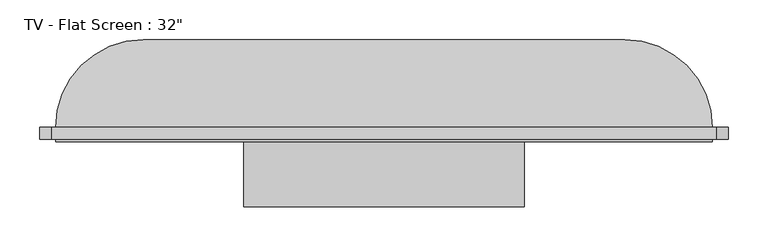
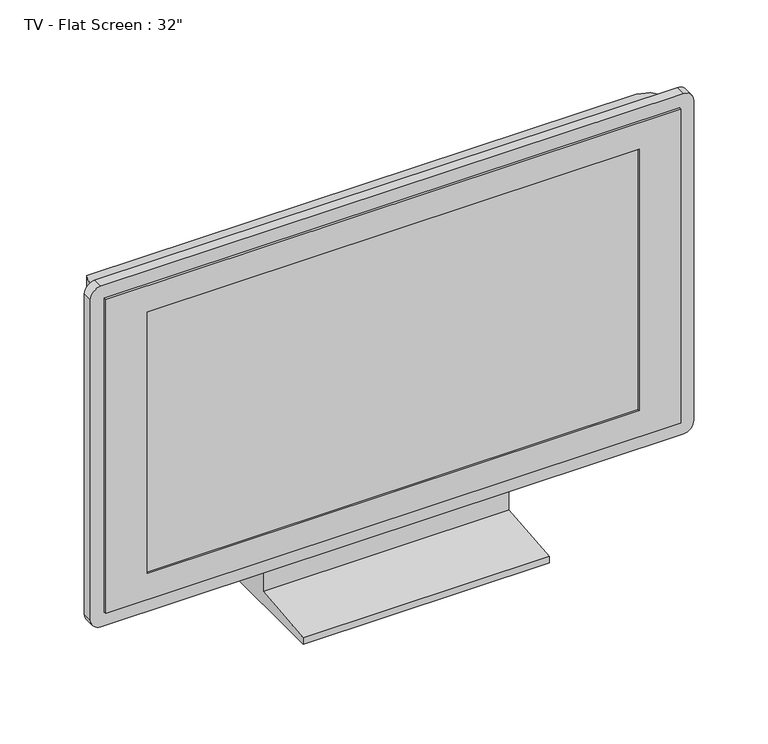
"""IFC4 building model written with IfcOpenShell, lengths in millimetres: furniture geometry."""

from ifc_helpers import new_model, si_unit, point, frame, frame_2d, origin, place, context, project, spatial, polyline, circle_curve, ellipse_curve, trimmed, segment, composite_curve, outline, extrude, faceted_brep, source, transform, mapped, element, save
from ifc_brep_helpers import plane_surface, cylinder_surface, advanced_brep


def furniture_56245f3a(model_context):
    return source(origin(), model_context, "Body", "SolidModel", [
        extrude(outline(polyline([(-51.4613764, 80.0), (-1.4613764, 80.0), (48.5386236, 0.0), (-151.4613764, 0.0), (-151.4613764, 10.0), (-51.4613764, 20.0), (-51.4613764, 80.0)])), frame((-180.4346678, 0.0, 0.0), z_axis=(1.0, 0.0, 0.0), x_axis=(0.0, 1.0, 0.0)), (0.0, 0.0, 1.0), 352.9803073),
        faceted_brep([(409.0357931, -69.4613764, 557.1392838), (-416.9248214, -69.4613764, 557.1392838), (-416.9248214, -69.4613764, 80.0), (409.0357931, -69.4613764, 80.0), (-356.9248214, -69.4613764, 517.1392838), (349.0357931, -69.4613764, 517.1392838), (349.0357931, -69.4613764, 120.0), (-356.9248214, -69.4613764, 120.0), (409.0357931, -51.4613764, 557.1392838), (409.0357931, -51.4613764, 80.0), (-416.9248214, -51.4613764, 80.0), (-416.9248214, -51.4613764, 557.1392838), (-356.9248214, -66.4613764, 517.1392838), (-356.9248214, -66.4613764, 120.0), (349.0357931, -66.4613764, 120.0), (349.0357931, -66.4613764, 517.1392838)], [[[0, 1, 2, 3], [4, 5, 6, 7]], [[8, 9, 10, 11]], [[1, 0, 8, 11]], [[2, 1, 11, 10]], [[3, 2, 10, 9]], [[0, 3, 9, 8]], [[12, 13, 14, 15]], [[12, 15, 5, 4]], [[15, 14, 6, 5]], [[14, 13, 7, 6]], [[13, 12, 4, 7]]]),
        extrude(outline(composite_curve([segment(polyline([(577.1392838, 414.0357931), (577.1392838, -421.9248214)]), True, "CONTINUOUS"), segment(trimmed(circle_curve(frame_2d((562.1392838, -421.9248214)), 15.0), [point((577.1392838, -421.9248214))], [point((562.1392838, -436.9248214))], False, "CARTESIAN"), True, "CONTINUOUS"), segment(polyline([(562.1392838, -436.9248214), (75.0, -436.9248214)]), True, "CONTINUOUS"), segment(trimmed(circle_curve(frame_2d((75.0, -421.9248214)), 15.0), [point((75.0, -436.9248214))], [point((60.0, -421.9248214))], False, "CARTESIAN"), True, "CONTINUOUS"), segment(polyline([(60.0, -421.9248214), (60.0, 414.0357931)]), True, "CONTINUOUS"), segment(trimmed(circle_curve(frame_2d((75.0, 414.0357931)), 15.0), [point((60.0, 414.0357931))], [point((75.0, 429.0357931))], False, "CARTESIAN"), True, "CONTINUOUS"), segment(polyline([(75.0, 429.0357931), (562.1392838, 429.0357931)]), True, "CONTINUOUS"), segment(trimmed(circle_curve(frame_2d((562.1392838, 414.0357931)), 15.0), [point((562.1392838, 429.0357931))], [point((577.1392838, 414.0357931))], False, "CARTESIAN"), True, "CONTINUOUS")], self_intersect=False), holes=[polyline([(557.1392838, 409.0357931), (80.0, 409.0357931), (80.0, -416.9248214), (557.1392838, -416.9248214), (557.1392838, 409.0357931)])]), frame((0.0, -66.4613764, 0.0), z_axis=(0.0, 1.0, 0.0), x_axis=(0.0, 0.0, 1.0)), (0.0, 0.0, 1.0), 15.0),
        advanced_brep(
        [(-416.9248214, -51.4613764, 80.0), (409.0357931, -51.4613764, 80.0), (409.0357931, -51.4613764, 557.1392838), (-416.9248214, -51.4613764, 557.1392838), (299.0357931, 58.5386236, 80.0), (-306.9248214, 58.5386236, 80.0), (-306.9248214, 58.5386236, 447.1392838), (299.0357931, 58.5386236, 447.1392838)],
        [
            (0, 1),
            (1, 2),
            (2, 3),
            (3, 0),
            (4, 5),
            (5, 6),
            (6, 7),
            (7, 4),
            (0, 5, circle_curve(frame((-306.9248214, -51.4613764, 80.0), z_axis=(0.0, 0.0, -1.0), x_axis=(-1.0, 0.0, 0.0)), 110.0)),
            (4, 1, circle_curve(frame((299.0357931, -51.4613764, 80.0), z_axis=(0.0, 0.0, -1.0), x_axis=(1.0, 0.0, 0.0)), 110.0)),
            (7, 2, ellipse_curve(frame((299.0357931, -51.4613764, 447.1392838), z_axis=(0.7071067811865475, 0.0, -0.7071067811865475), x_axis=(0.7071067811865474, 0.0, 0.7071067811865476)), 155.5634919, 110.0)),
            (6, 3, ellipse_curve(frame((-306.9248214, -51.4613764, 447.1392838), z_axis=(0.7071067811865475, 0.0, 0.7071067811865475), x_axis=(-0.7071067811865476, 0.0, 0.7071067811865474)), 155.5634919, 110.0)),
        ],
        [
            plane_surface(frame((-416.9248214, -51.4613764, 557.1392838), z_axis=(0.0, -1.0, 0.0), x_axis=(-1.0, 0.0, 0.0))),
            plane_surface(frame((-416.9248214, 58.5386236, 557.1392838), z_axis=(0.0, 1.0, 0.0), x_axis=(1.0, 0.0, 0.0))),
            plane_surface(frame((-416.9248214, -51.4613764, 80.0), z_axis=(0.0, 0.0, -1.0), x_axis=(0.0, 1.0, 0.0))),
            cylinder_surface(frame((299.0357931, -51.4613764, 80.0), z_axis=(0.0, 0.0, 1.0), x_axis=(1.0, 0.0, 0.0)), 110.0),
            cylinder_surface(frame((409.0357931, -51.4613764, 447.1392838), z_axis=(-1.0, 0.0, 0.0), x_axis=(0.0, 0.0, 1.0)), 110.0),
            cylinder_surface(frame((-306.9248214, -51.4613764, 557.1392838), z_axis=(0.0, 0.0, -1.0), x_axis=(-1.0, 0.0, 0.0)), 110.0),
        ],
        [
            (0, [[1, 2, 3, 4]]),
            (1, [[5, 6, 7, 8]]),
            (2, [[-1, 9, -5, 10]]),
            (3, [[11, -2, -10, -8]]),
            (4, [[-11, -7, 12, -3]]),
            (5, [[-12, -6, -9, -4]]),
        ],
    ),
    ])


if __name__ == "__main__":
    model = new_model("IFC4")
    model_context = context("Model", 3, world=origin())
    ifc_project = project(units=[si_unit("LENGTHUNIT", "METRE", prefix="MILLI")], contexts=[model_context])
    site = spatial("IfcSite", under=ifc_project)
    building = spatial("IfcBuilding", under=site)
    placement = place(None, origin())
    furniture_shape = furniture_56245f3a(model_context)
    element("IfcFurniture", 1, ObjectType="TV - Flat Screen : 32\"", at=placement, inside=building, context=model_context, shape_type="MappedRepresentation", body=[
        mapped(furniture_shape, transform((0.0, 0.0, 0.0), x_axis=(1.0, 0.0, 0.0), y_axis=(0.0, 1.0, 0.0), z_axis=(0.0, 0.0, 1.0))),
    ])
    save(model, "model.ifc")

# Revit data of these elements
# Type "TV - Flat Screen : 32\""
#   SinAng = 0' - 0.0193"
#   L = 2' - 3.79372"
#   H = 1' - 3.6354"
#   Thickness = 0' - 4.33071"
#   Diagonal = 2' - 7.88976"
#   CosAng = 0' - 0.03431"
#   Stand [instance default] = yes
# Element 1 (IfcFurniture, "TV - Flat Screen : 32\"")
#   Materials on its faces: "TV - Black", "TV - Glass", "TV - Screen"
# Materials
#   "TV - Black": colour RGB 49 49 49, transparency 0
#   "TV - Glass": colour RGB 157 157 157, transparency 0.9
#   "TV - Screen": colour RGB 0 0 0, transparency 0
